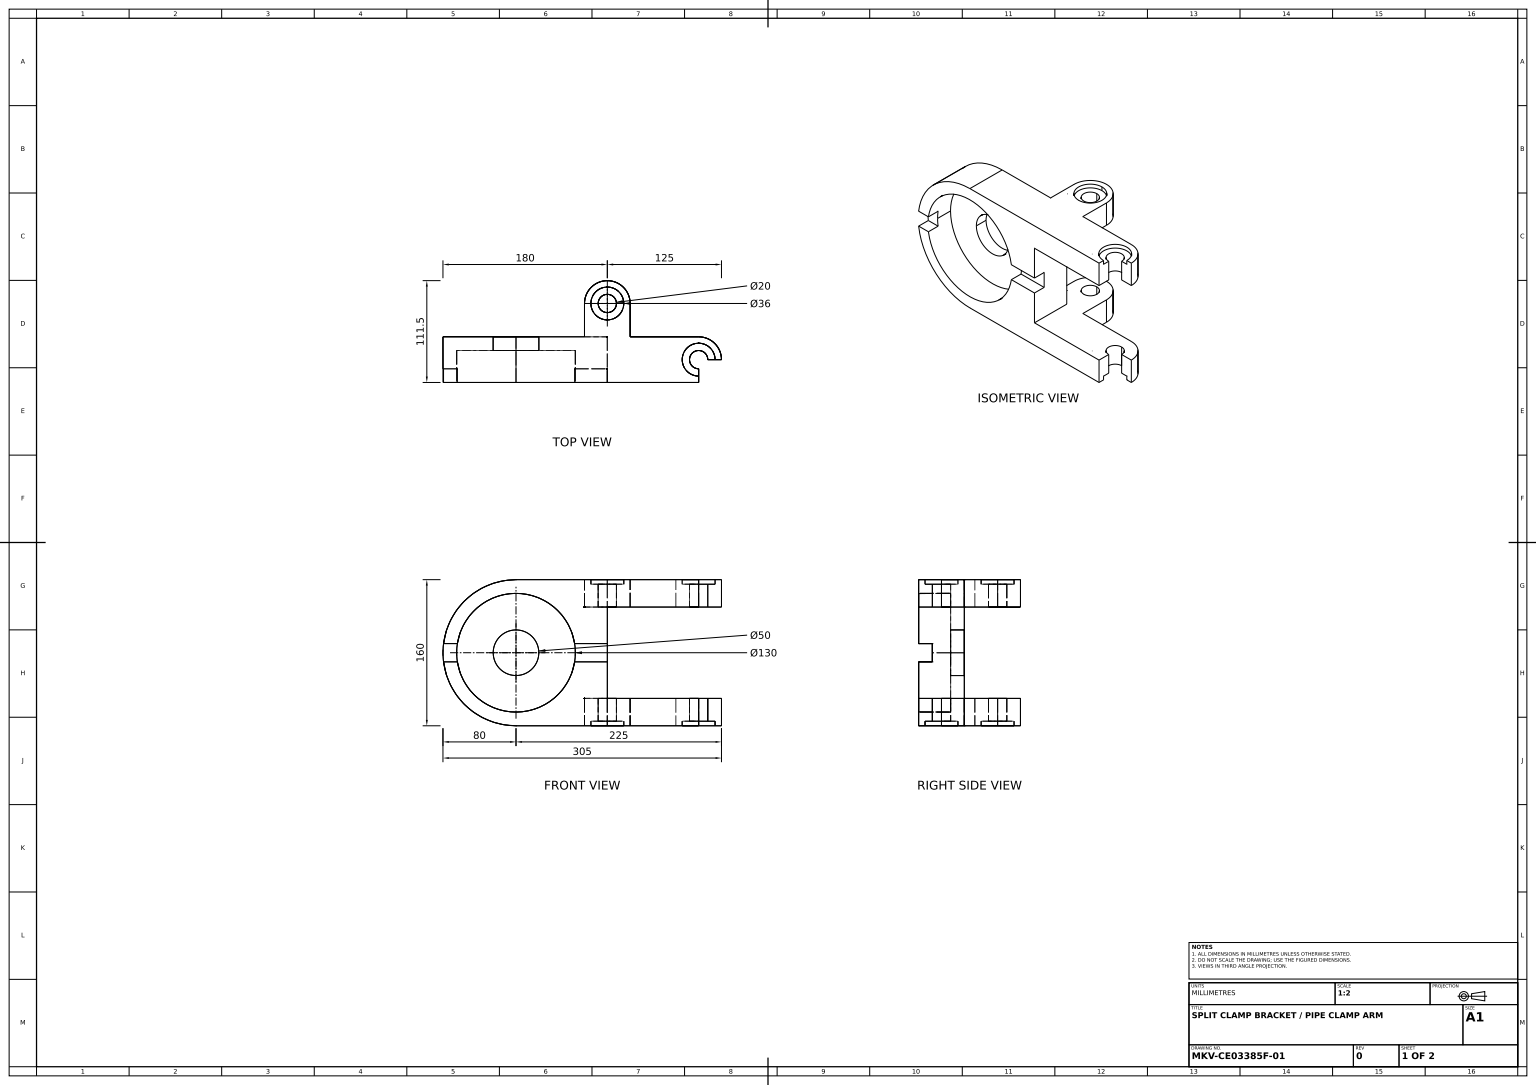
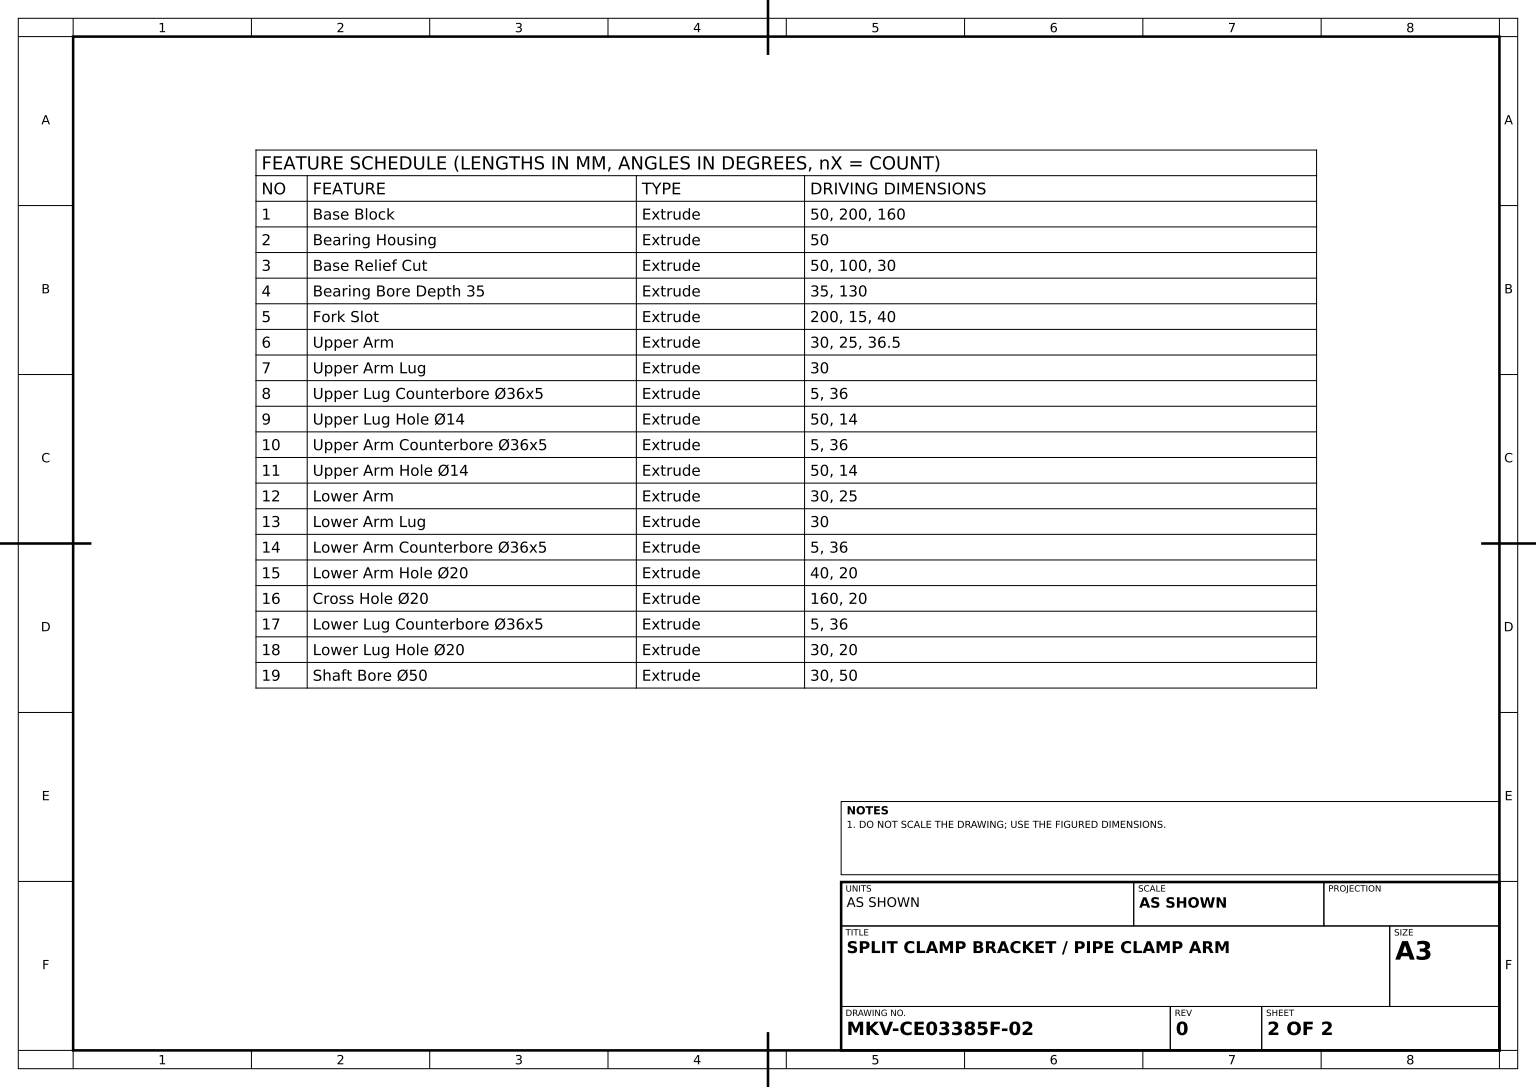
from build123d import *

# Parameters (mm, degrees)
BASE_BLOCK_SKETCH_W              = 200
BASE_BLOCK_SKETCH_H              = 160
BASE_BLOCK_DEPTH                 = 50
BEARING_HOUSING_DEPTH            = 50
BASE_RELIEF_CUT_SKETCH_W         = 100
BASE_RELIEF_CUT_SKETCH_H         = 100
BASE_RELIEF_CUT_DEPTH            = 50
BEARING_BORE_SKETCH_R            = 65
BEARING_BORE_DEPTH_35_DEPTH      = 35
FORK_SLOT_DEPTH                  = 200
UPPER_ARM_DEPTH                  = 30
UPPER_START                      = -30
UPPER_ARM_LUG_DEPTH              = 30
UPPER_LUG_COUNTERBORE_SKETCH_R   = 18
UPPER_LUG_COUNTERBORE_36X5_DEPTH = 5
UPPER_LUG_HOLE_SKETCH_R          = 7
UPPER_LUG_HOLE_14_DEPTH          = 50
UPPER_START_2                    = -5
UPPER_ARM_COUNTERBORE_SKETCH_R   = 18
UPPER_ARM_COUNTERBORE_36X5_DEPTH = 5
UPPER_START_3                    = -50
UPPER_ARM_HOLE_SKETCH_R          = 7
UPPER_ARM_HOLE_14_DEPTH          = 50
LOWER_ARM_DEPTH                  = 30
LOWER_START                      = -30
LOWER_ARM_LUG_DEPTH              = 30
LOWER_ARM_COUNTERBORE_SKETCH_R   = 18
LOWER_ARM_COUNTERBORE_36X5_DEPTH = 5
LOWER_ARM_HOLE_SKETCH_R          = 10
LOWER_ARM_HOLE_20_DEPTH          = 40
CROSS_HOLE_SKETCH_R              = 10
CROSS_HOLE_20_DEPTH              = 160
LOWER_START_2                    = -5
LOWER_LUG_COUNTERBORE_SKETCH_R   = 18
LOWER_LUG_COUNTERBORE_36X5_DEPTH = 5
LOWER_LUG_HOLE_SKETCH_R          = 10
LOWER_LUG_HOLE_20_DEPTH          = 30
SHAFT_BORE_SKETCH_R              = 25
SHAFT_BORE_50_DEPTH              = 30


with BuildPart() as part:
    # Base Block Sketch → Base Block (new body)
    with BuildSketch(Plane.XY):
        with Locations((100, 80)):
            Rectangle(BASE_BLOCK_SKETCH_W, BASE_BLOCK_SKETCH_H)
    extrude(amount=BASE_BLOCK_DEPTH)

    # Bearing Housing Sketch → Bearing Housing (add)
    with BuildSketch(Plane.XY.offset(50)):
        with BuildLine():
            Line((0, 160), (0, 0))
            ThreePointArc((0, 0), (-80, 80), (0, 160))
        make_face()
    extrude(amount=-BEARING_HOUSING_DEPTH)

    # Base Relief Cut Sketch → Base Relief Cut (cut)
    with BuildSketch(Plane.XY.offset(50)):
        with Locations((150, 80)):
            Rectangle(BASE_RELIEF_CUT_SKETCH_W, BASE_RELIEF_CUT_SKETCH_H)
    extrude(amount=-BASE_RELIEF_CUT_DEPTH, mode=Mode.SUBTRACT)

    # Bearing Bore Sketch → Bearing Bore Depth 35 (cut)
    with BuildSketch(Plane.XY.offset(50)):
        with Locations((0, 80)):
            Circle(BEARING_BORE_SKETCH_R)
    extrude(amount=-BEARING_BORE_DEPTH_35_DEPTH, mode=Mode.SUBTRACT)

    # Fork Slot Sketch → Fork Slot (cut)
    with BuildSketch(Plane(origin=(100, 0, 0), x_dir=(0, 0, -1), z_dir=(1, 0, 0))):
        Polygon((-50, 80), (-50, 90), (-35, 90), (-35, 70), (-50, 70), align=None)
    extrude(amount=-FORK_SLOT_DEPTH, mode=Mode.SUBTRACT)

    # Upper Arm Sketch → Upper Arm (add)
    with BuildSketch(Plane.XZ):
        with BuildLine():
            Line((125, 0), (100, 0))
            Line((100, 0), (75, 0))
            Line((75, 0), (75, -36.5))
            ThreePointArc((75, -36.5), (100, -61.5), (125, -36.5))
            Line((125, -36.5), (125, 0))
        make_face()
    extrude(amount=-UPPER_ARM_DEPTH)

    # Upper Arm Lug Sketch → Upper Arm Lug (add)
    with BuildSketch(Plane(origin=(0, 160, 0), x_dir=(1, 0, 0), z_dir=(0, 1, 0)).offset(UPPER_START)):
        with BuildLine():
            Line((75, 36.5), (75, 0))
            Line((75, 0), (125, 0))
            Line((125, 0), (125, 36.5))
            ThreePointArc((125, 36.5), (100, 61.5), (75, 36.5))
        make_face()
    extrude(amount=UPPER_ARM_LUG_DEPTH)

    # Upper Lug Counterbore Sketch → Upper Lug Counterbore Ø36x5 (cut)
    with BuildSketch(Plane(origin=(0, 160, 0), x_dir=(1, 0, 0), z_dir=(0, 1, 0))):
        with Locations(Location((100, 36.5, 0), (0, 0, 270))):
            Circle(UPPER_LUG_COUNTERBORE_SKETCH_R)
    extrude(amount=-UPPER_LUG_COUNTERBORE_36X5_DEPTH, mode=Mode.SUBTRACT)

    # Upper Lug Hole Sketch → Upper Lug Hole Ø14 (cut)
    with BuildSketch(Plane(origin=(0, 155, 0), x_dir=(1, 0, 0), z_dir=(0, 1, 0))):
        with Locations(Location((100, 36.5, 0), (0, 0, 270))):
            Circle(UPPER_LUG_HOLE_SKETCH_R)
    extrude(amount=-UPPER_LUG_HOLE_14_DEPTH, mode=Mode.SUBTRACT)

    # Upper Arm Counterbore Sketch → Upper Arm Counterbore Ø36x5 (cut)
    with BuildSketch(Plane.XZ.offset(UPPER_START_2)):
        with Locations(Location((100, -36.5, 0), (0, 0, 90))):
            Circle(UPPER_ARM_COUNTERBORE_SKETCH_R)
    extrude(amount=UPPER_ARM_COUNTERBORE_36X5_DEPTH, mode=Mode.SUBTRACT)

    # Upper Arm Hole Sketch → Upper Arm Hole Ø14 (cut)
    with BuildSketch(Plane.XZ.offset(-5).offset(UPPER_START_3)):
        with Locations(Location((100, -36.5, 0), (0, 0, 90))):
            Circle(UPPER_ARM_HOLE_SKETCH_R)
    extrude(amount=UPPER_ARM_HOLE_14_DEPTH, mode=Mode.SUBTRACT)

    # Lower Arm Sketch → Lower Arm (add)
    with BuildSketch(Plane.XZ):
        with BuildLine():
            Line((225, 25), (200, 25))
            Line((200, 25), (200, 50))
            ThreePointArc((200, 50), (182.32233047, 7.32233047), (225, 25))
        make_face()
    extrude(amount=-LOWER_ARM_DEPTH)

    # Lower Arm Lug Sketch → Lower Arm Lug (add)
    with BuildSketch(Plane(origin=(0, 160, 0), x_dir=(1, 0, 0), z_dir=(0, 1, 0)).offset(LOWER_START)):
        with BuildLine():
            Line((200, -25), (225, -25))
            ThreePointArc((225, -25), (217.67766953, -7.32233047), (200, 0))
            Line((200, 0), (200, -25))
        make_face()
    extrude(amount=LOWER_ARM_LUG_DEPTH)

    # Lower Arm Counterbore Sketch → Lower Arm Counterbore Ø36x5 (cut)
    with BuildSketch(Plane.XZ):
        with Locations((200, 25)):
            Circle(LOWER_ARM_COUNTERBORE_SKETCH_R)
    extrude(amount=-LOWER_ARM_COUNTERBORE_36X5_DEPTH, mode=Mode.SUBTRACT)

    # Lower Arm Hole Sketch → Lower Arm Hole Ø20 (cut)
    with BuildSketch(Plane.XZ.offset(-5)):
        with Locations((200, 25)):
            Circle(LOWER_ARM_HOLE_SKETCH_R)
    extrude(amount=-LOWER_ARM_HOLE_20_DEPTH, mode=Mode.SUBTRACT)

    # Cross Hole Sketch → Cross Hole Ø20 (cut)
    with BuildSketch(Plane.XZ.offset(-5)):
        with Locations(Location((100, -36.5, 0), (0, 0, 270))):
            Circle(CROSS_HOLE_SKETCH_R)
    extrude(amount=-CROSS_HOLE_20_DEPTH, mode=Mode.SUBTRACT)

    # Lower Lug Counterbore Sketch → Lower Lug Counterbore Ø36x5 (cut)
    with BuildSketch(Plane(origin=(0, 160, 0), x_dir=(1, 0, 0), z_dir=(0, 1, 0)).offset(LOWER_START_2)):
        with Locations((200, -25)):
            Circle(LOWER_LUG_COUNTERBORE_SKETCH_R)
    extrude(amount=LOWER_LUG_COUNTERBORE_36X5_DEPTH, mode=Mode.SUBTRACT)

    # Lower Lug Hole Sketch → Lower Lug Hole Ø20 (cut)
    with BuildSketch(Plane(origin=(0, 160, 0), x_dir=(1, 0, 0), z_dir=(0, 1, 0)).offset(LOWER_START)):
        with Locations((200, -25)):
            Circle(LOWER_LUG_HOLE_SKETCH_R)
    extrude(amount=LOWER_LUG_HOLE_20_DEPTH, mode=Mode.SUBTRACT)

    # Shaft Bore Sketch → Shaft Bore Ø50 (cut)
    with BuildSketch(Plane.XY.offset(15)):
        with Locations((0, 80)):
            Circle(SHAFT_BORE_SKETCH_R)
    extrude(amount=-SHAFT_BORE_50_DEPTH, mode=Mode.SUBTRACT)


solid = part.part
